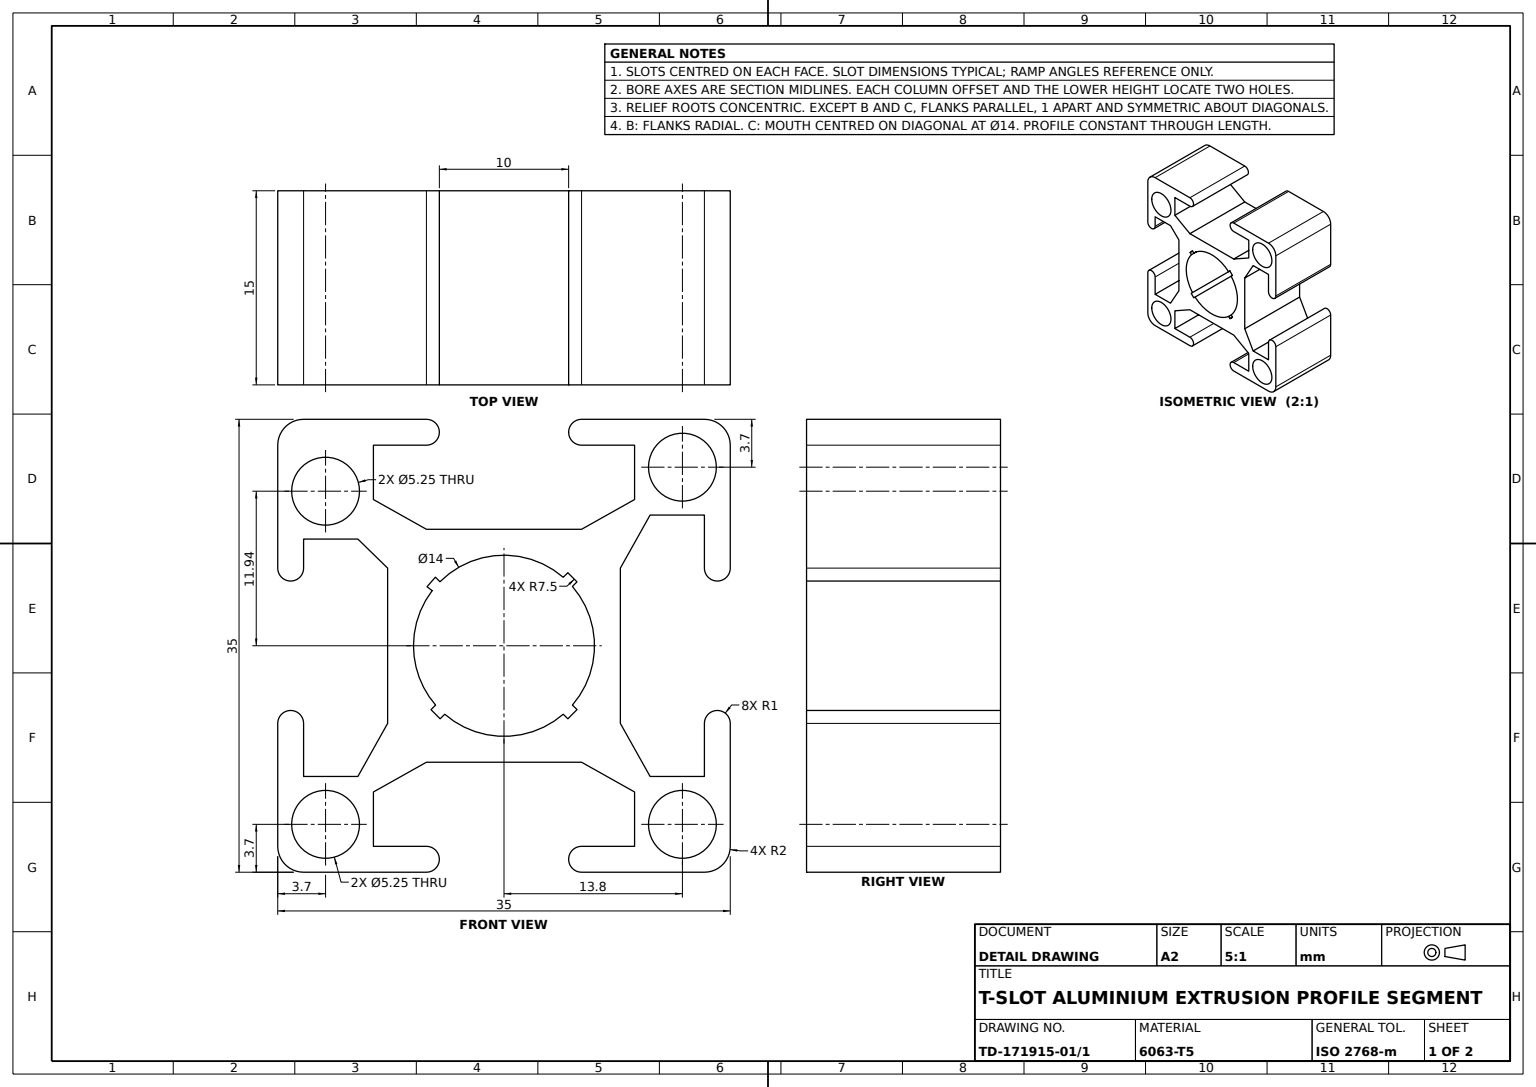
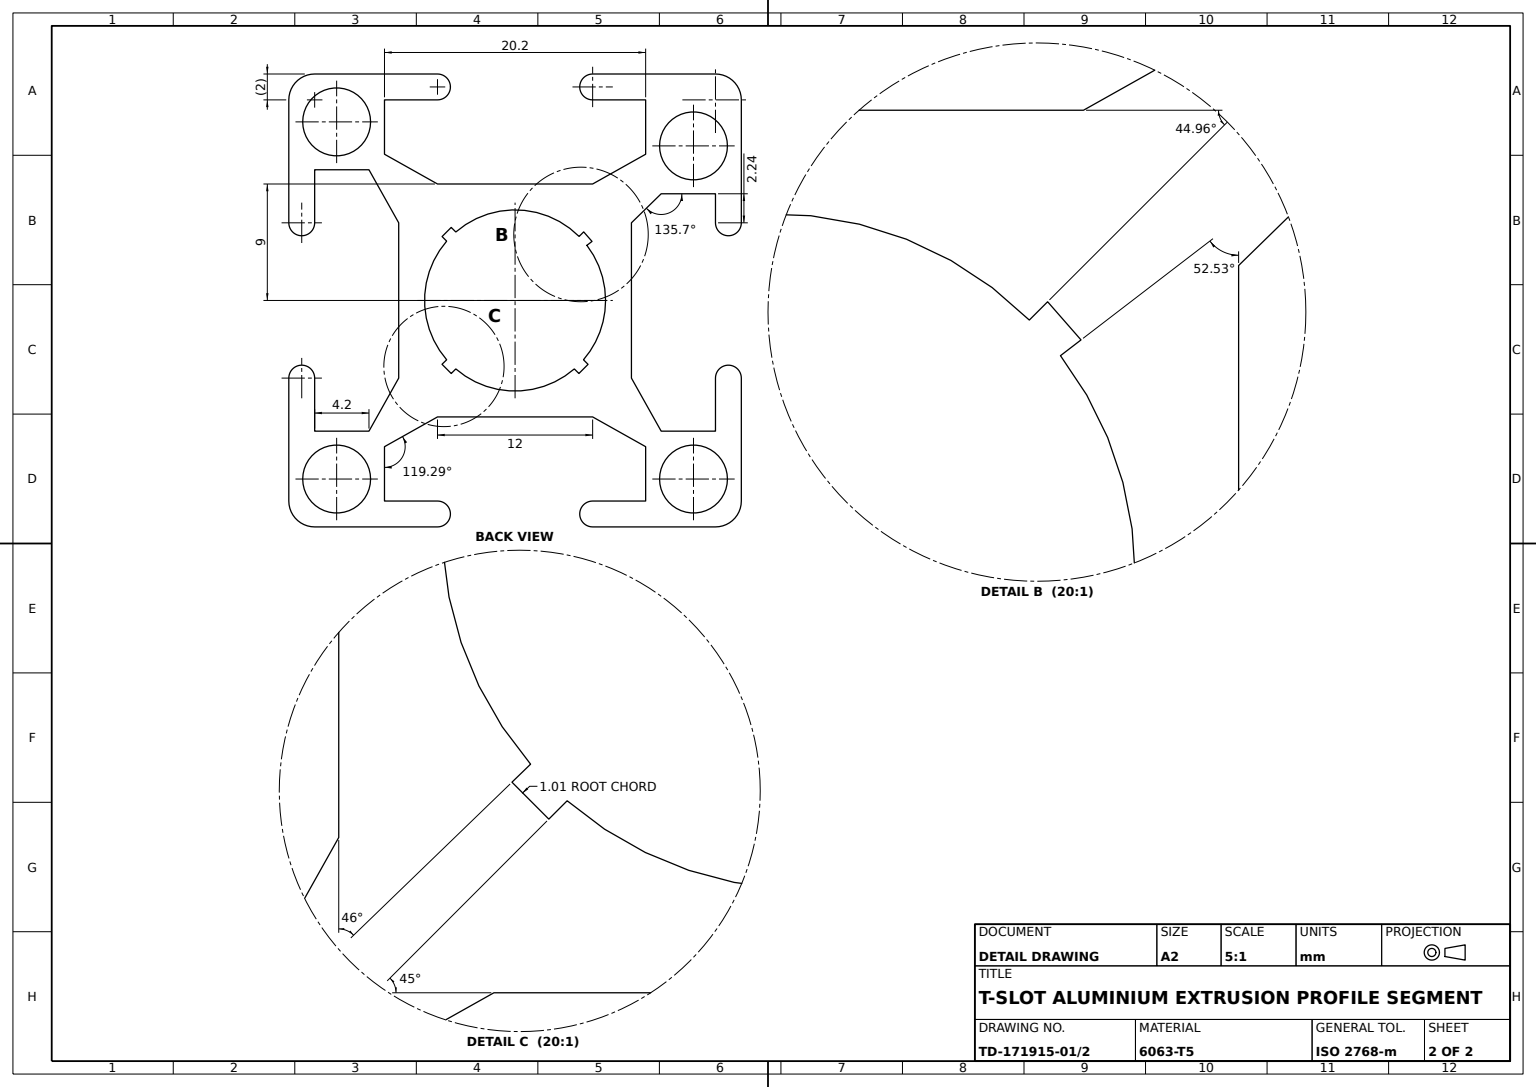
from build123d import *

# Parameters (mm, degrees)
PROFILE_SECTION_35X35_R     = 2.625
PROFILE_EXTRUSION_L15_DEPTH = 7.5


with BuildPart() as part:
    # Profile Section 35x35 → Profile Extrusion L15 (new, symmetric)
    with BuildSketch(Plane.XY):
        with BuildLine():
            Line((-13.8, -17.5), (-6, -17.5))
            ThreePointArc((-6, -17.5), (-5, -16.5), (-6, -15.5))
            Line((-6, -15.5), (-10.1, -15.5))
            Line((-10.1, -15.5), (-10.1, -11.3))
            Line((-10.1, -11.3), (-6, -9))
            Line((-6, -9), (0, -9))
            Line((0, -9), (6, -9))
            Line((6, -9), (10.1, -11.3))
            Line((10.1, -11.3), (10.1, -15.5))
            Line((10.1, -15.5), (6, -15.5))
            ThreePointArc((6, -15.5), (5, -16.5), (6, -17.5))
            Line((6, -17.5), (13.8, -17.5))
            Line((13.8, -17.5), (15.5, -17.5))
            ThreePointArc((15.5, -17.5), (16.914213562, -16.914213562), (17.5, -15.5))
            Line((17.5, -15.5), (17.5, -6))
            ThreePointArc((17.5, -6), (16.5, -5), (15.5, -6))
            Line((15.5, -6), (15.5, -10.1))
            Line((15.5, -10.1), (11.3, -10.1))
            Line((11.3, -10.1), (9, -6))
            Line((9, -6), (9, 0))
            Line((9, 0), (9, 6))
            Line((9, 6), (11.3, 10.1))
            Line((11.3, 10.1), (15.5, 10.1))
            Line((15.5, 10.1), (15.5, 6))
            ThreePointArc((15.5, 6), (16.5, 5), (17.5, 6))
            Line((17.5, 6), (17.5, 15.5))
            ThreePointArc((17.5, 15.5), (16.914213562, 16.914213562), (15.5, 17.5))
            Line((15.5, 17.5), (13.8, 17.5))
            Line((13.8, 17.5), (6, 17.5))
            ThreePointArc((6, 17.5), (5, 16.5), (6, 15.5))
            Line((6, 15.5), (10.1, 15.5))
            Line((10.1, 15.5), (10.1, 11.3))
            Line((10.1, 11.3), (6, 9))
            Line((6, 9), (0, 9))
            Line((0, 9), (-6, 9))
            Line((-6, 9), (-10.1, 11.3))
            Line((-10.1, 11.3), (-10.1, 15.5))
            Line((-10.1, 15.5), (-6, 15.5))
            ThreePointArc((-6, 15.5), (-5, 16.5), (-6, 17.5))
            Line((-6, 17.5), (-13.8, 17.5))
            Line((-13.8, 17.5), (-15.5, 17.5))
            ThreePointArc((-15.5, 17.5), (-16.914213562, 16.914213562), (-17.5, 15.5))
            Line((-17.5, 15.5), (-17.5, 6))
            ThreePointArc((-17.5, 6), (-16.5, 5), (-15.5, 6))
            Line((-15.5, 6), (-15.5, 8.244179001))
            Line((-15.5, 8.244179001), (-11.3, 8.244179001))
            Line((-11.3, 8.244179001), (-9, 6))
            Line((-9, 6), (-9, 0))
            Line((-9, 0), (-9, -6))
            Line((-9, -6), (-11.3, -10.1))
            Line((-11.3, -10.1), (-15.5, -10.1))
            Line((-15.5, -10.1), (-15.5, -6))
            ThreePointArc((-15.5, -6), (-16.5, -5), (-17.5, -6))
            Line((-17.5, -6), (-17.5, -15.5))
            ThreePointArc((-17.5, -15.5), (-16.914213562, -16.914213562), (-15.5, -17.5))
            Line((-15.5, -17.5), (-13.8, -17.5))
        make_face()
        with Locations((-13.8, -13.8)):
            Circle(PROFILE_SECTION_35X35_R, mode=Mode.SUBTRACT)
        with Locations((13.8, -13.8)):
            Circle(PROFILE_SECTION_35X35_R, mode=Mode.SUBTRACT)
        with Locations((-13.8, 11.944179001)):
            Circle(PROFILE_SECTION_35X35_R, mode=Mode.SUBTRACT)
        with BuildLine():
            Line((5.645056013, 4.937949232), (5.290657805, 4.583551024))
            ThreePointArc((5.290657805, 4.583551024), (6.999999998, -0.000156062), (5.290453424, -4.583786925))
            Line((5.290453424, -4.583786925), (5.650606112, -4.931597162))
            ThreePointArc((5.650606112, -4.931597162), (5.30628231, -5.300317731), (4.937949232, -5.645056013))
            Line((4.937949232, -5.645056013), (4.583551024, -5.290657805))
            ThreePointArc((4.583551024, -5.290657805), (0, -7), (-4.583551024, -5.290657805))
            Line((-4.583551024, -5.290657805), (-4.937949232, -5.645056013))
            ThreePointArc((-4.937949232, -5.645056013), (-5.303300859, -5.303300859), (-5.645056013, -4.937949232))
            Line((-5.645056013, -4.937949232), (-5.290657805, -4.583551024))
            ThreePointArc((-5.290657805, -4.583551024), (-6.996859079, -0.209673625), (-5.555626638, 4.258522357))
            Line((-5.555626638, 4.258522357), (-5.952457112, 4.562702525))
            ThreePointArc((-5.952457112, 4.562702525), (-5.64166709, 4.941820762), (-5.306773753, 5.299825689))
            Line((-5.306773753, 5.299825689), (-4.952988836, 4.946503977))
            ThreePointArc((-4.952988836, 4.946503977), (-0.252451062, 6.995446266), (4.583551024, 5.290657805))
            Line((4.583551024, 5.290657805), (4.937949232, 5.645056013))
            ThreePointArc((4.937949232, 5.645056013), (5.303300859, 5.303300859), (5.645056013, 4.937949232))
        make_face(mode=Mode.SUBTRACT)
        with Locations((13.8, 13.8)):
            Circle(PROFILE_SECTION_35X35_R, mode=Mode.SUBTRACT)
    extrude(amount=PROFILE_EXTRUSION_L15_DEPTH, both=True)


solid = part.part
